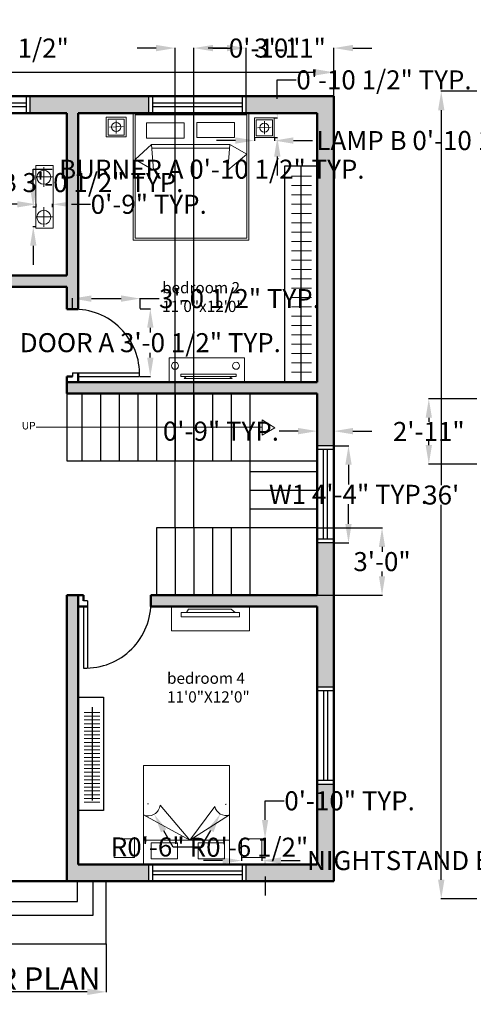
# Model space of a CAD drawing. Units: inches. Extents: x 18 to 9768, y 4 to 3529.
# Tile 3 of 6: x 9006 to 9249, y 3002 to 3529. Entities that reach past the tile are written whole.
import ezdxf

# ---------------------------------------------------------------- set-up
doc = ezdxf.new("R2010")
doc.units = ezdxf.units.IN
doc.header["$MEASUREMENT"] = 0
for name, color, linetype, lineweight in [('A-ANNO-DIMS', 2, 'Continuous', 18), ('A-ANNO-SYMB', 2, 'Continuous', 18), ('A-ANNO-TEXT', 7, 'Continuous', 25), ('A-AREA-IDEN', 7, 'Continuous', 18), ('A-CASE-PATT', 9, 'Continuous', 13), ('A-EQPM', 8, 'Continuous', 18), ('A-FLOR-CASE', 9, 'Continuous', 25), ('A-FLOR-STRS', 7, 'Continuous', 25), ('A-FURN', 8, 'Continuous', 18), ('A-WALL-PATT', 252, 'Continuous', 13), ('WAL', 7, 'Continuous', 50)]:
    doc.layers.add(name, color=color, linetype=linetype, lineweight=lineweight)
doc.layers.add('A-DOOR', color=30, linetype='Continuous', lineweight=25, true_color=0xf8991e)
doc.layers.add('A-GLAZ', color=177, linetype='Continuous', lineweight=25, true_color=0x293189)
doc.styles.get("Standard").update_dxf_attribs({"font": 'arial.ttf'})
doc.dimstyles.get("Standard").update_dxf_attribs({"dimtxt": 10.18, "dimasz": 10.18, "dimexe": 0.18, "dimexo": 0.0625, "dimgap": 0.09, "dimtad": 0, "dimtih": 1, "dimtoh": 1, "dimdec": 0, "dimzin": 0, "dimdsep": 46, "dimlunit": 3, "dimtxsty": 'Standard', "dimcen": 0.09, "dimadec": 0, "dimazin": 0, "dimtfac": 1, "dimtdec": 0, "dimtofl": 0, "dimtmove": 0, "dimatfit": 3, "dimfxl": 1, "dimtolj": 1, "dimtzin": 0, "dimarcsym": 0})

# ---------------------------------------------------------------- blocks, each defined once
blk = doc.blocks.new('*D3')
at = {"layer": 'A-ANNO-DIMS', "color": 0, "lineweight": -2, "transparency": 16777216}
for p, q in [((8753.89, 3487.8), (8753.89, 3500.68)), ((8764.07, 3500.5), (8955.16, 3500.5)), ((9163.71, 3500.5), (8972.61, 3500.5)), ((9173.89, 3487.8), (9173.89, 3500.68))]:
    blk.add_line(p, q, dxfattribs=at)
at = {"layer": 'A-ANNO-DIMS', "color": 0, "transparency": 16777216}
for points in [[(8764.07, 3502.19), (8764.07, 3498.8), (8753.89, 3500.5)], [(9163.71, 3502.19), (9163.71, 3498.8), (9173.89, 3500.5)]]:
    blk.add_solid(points, dxfattribs=at)
at = {"layer": 'Defpoints', "color": 0, "transparency": 16777216}
for p in [(9173.89, 3500.5), (8753.89, 3487.73), (9173.89, 3487.73)]:
    blk.add_point(p, dxfattribs=at)
at = {"layer": 'A-ANNO-DIMS', "color": 0, "transparency": 16777216, "insert": (8963.89, 3500.5), "char_height": 10.18, "attachment_point": 5}
blk.add_mtext("\\A1;35'", dxfattribs=at)
blk = doc.blocks.new('*D8')
at = {"layer": 'A-ANNO-DIMS', "color": 0, "lineweight": -2, "transparency": 16777216}
for p, q in [((9250.37, 3490.36), (9231.16, 3490.36)), ((9231.34, 3480.18), (9231.34, 3279.65)), ((9231.34, 3068.54), (9231.34, 3269.07)), ((9250.37, 3058.36), (9231.16, 3058.36))]:
    blk.add_line(p, q, dxfattribs=at)
at = {"layer": 'A-ANNO-DIMS', "color": 0, "transparency": 16777216}
for points in [[(9229.65, 3480.18), (9233.04, 3480.18), (9231.34, 3490.36)], [(9229.65, 3068.54), (9233.04, 3068.54), (9231.34, 3058.36)]]:
    blk.add_solid(points, dxfattribs=at)
at = {"layer": 'Defpoints', "color": 0, "transparency": 16777216}
for p in [(9250.43, 3490.36), (9231.34, 3058.36), (9250.43, 3058.36)]:
    blk.add_point(p, dxfattribs=at)
at = {"layer": 'A-ANNO-DIMS', "color": 0, "transparency": 16777216, "insert": (9231.34, 3274.36), "char_height": 10.18, "attachment_point": 5}
blk.add_mtext("\\A1;36'", dxfattribs=at)
blk = doc.blocks.new('WINDOW-48')
for p, q in [((0, 0), (0, 9)), ((2, 0), (2, 9)), ((2, 5.5), (50, 5.5)), ((50, 0), (50, 9)), ((52, 0), (52, 9)), ((2, 3.5), (50, 3.5))]:
    blk.add_line(p, q)
blk = doc.blocks.new('DOOR-36-W6')
for p, q in [((34.01, 0), (34.01, 36)), ((36.01, 3), (36.01, 36)), ((34.01, 0), (36.01, 0))]:
    blk.add_line(p, q)
blk.add_arc((35.01, 1), 35.01, 88.3634, 181.6366)
blk = doc.blocks.new('NIGHTSTAND-LAMP-B')
for p, q in [((1.67, 5.25), (8.97, 5.48)), ((5.32, 8.7), (5.32, 1.86))]:
    blk.add_line(p, q)
for points in [[(0, 10.5), (10.63, 10.5), (10.63, 0), (0, 0)], [(1, 9.5), (9.63, 9.5), (9.63, 1), (1, 1)]]:
    blk.add_lwpolyline(points, close=True)
blk.add_circle((5.32, 5.25), 2.45)
blk = doc.blocks.new('COOKTOP-BURNER-7')
for p, q in [((0, 5.3), (8.79, 5.3)), ((4.14, 10.42), (4.14, 0))]:
    blk.add_line(p, q)
blk.add_circle((4.08, 5.04), 3.73)
blk = doc.blocks.new('NIGHTSTAND-SMALL')
blk.add_lwpolyline([(0, 9.97), (10.94, 9.97), (10.94, 0), (0, 0)], close=True)
blk = doc.blocks.new('*D25')
at = {"layer": 'A-ANNO-DIMS', "color": 0, "lineweight": -2, "transparency": 16777216}
for p, q in [((9173.95, 3300.73), (9181.87, 3300.73)), ((9181.69, 3290.55), (9181.69, 3279.94)), ((9181.69, 3258.91), (9181.69, 3269.53)), ((9173.95, 3248.73), (9181.87, 3248.73))]:
    blk.add_line(p, q, dxfattribs=at)
at = {"layer": 'A-ANNO-DIMS', "color": 0, "transparency": 16777216}
for points in [[(9179.99, 3290.55), (9183.38, 3290.55), (9181.69, 3300.73)], [(9179.99, 3258.91), (9183.38, 3258.91), (9181.69, 3248.73)]]:
    blk.add_solid(points, dxfattribs=at)
at = {"layer": 'Defpoints', "color": 0, "transparency": 16777216}
for p in [(9173.89, 3300.73), (9181.69, 3300.73), (9173.89, 3248.73)]:
    blk.add_point(p, dxfattribs=at)
at = {"layer": 'A-ANNO-DIMS', "color": 0, "transparency": 16777216, "insert": (9181.69, 3274.73), "char_height": 10.18, "attachment_point": 5}
blk.add_mtext('\\A1;W1 4\'-4" TYP.', dxfattribs=at)
blk = doc.blocks.new('*D26')
at = {"layer": 'A-ANNO-DIMS', "color": 0, "lineweight": -2, "transparency": 16777216}
for p, q in [((9154.71, 3308.53), (9144.53, 3308.53)), ((9164.89, 3300.8), (9164.89, 3308.71)), ((9173.89, 3300.8), (9173.89, 3308.71)), ((9184.07, 3308.53), (9194.25, 3308.53))]:
    blk.add_line(p, q, dxfattribs=at)
at = {"layer": 'A-ANNO-DIMS', "color": 0, "transparency": 16777216}
for points in [[(9154.71, 3310.23), (9154.71, 3306.84), (9164.89, 3308.53)], [(9184.07, 3310.23), (9184.07, 3306.84), (9173.89, 3308.53)]]:
    blk.add_solid(points, dxfattribs=at)
at = {"layer": 'Defpoints', "color": 0, "transparency": 16777216}
for p in [(9164.89, 3308.53), (9164.89, 3300.73), (9173.89, 3300.73)]:
    blk.add_point(p, dxfattribs=at)
at = {"layer": 'A-ANNO-DIMS', "color": 0, "transparency": 16777216, "insert": (9113.41, 3308.53), "char_height": 10.18, "attachment_point": 5}
blk.add_mtext('\\A1;0\'-9" TYP.', dxfattribs=at)
blk = doc.blocks.new('*D29')
at = {"layer": 'A-ANNO-DIMS', "color": 0, "lineweight": -2, "transparency": 16777216}
for p, q in [((9070.22, 3374.01), (9075.78, 3374.01)), ((9075.6, 3363.83), (9075.6, 3361.23)), ((9075.6, 3347.91), (9075.6, 3350.51)), ((9070.22, 3337.73), (9075.78, 3337.73))]:
    blk.add_line(p, q, dxfattribs=at)
at = {"layer": 'A-ANNO-DIMS', "color": 0, "transparency": 16777216}
for points in [[(9073.9, 3363.83), (9077.3, 3363.83), (9075.6, 3374.01)], [(9073.9, 3347.91), (9077.3, 3347.91), (9075.6, 3337.73)]]:
    blk.add_solid(points, dxfattribs=at)
at = {"layer": 'Defpoints', "color": 0, "transparency": 16777216}
for p in [(9070.16, 3374.01), (9070.16, 3337.73), (9075.6, 3337.73)]:
    blk.add_point(p, dxfattribs=at)
at = {"layer": 'A-ANNO-DIMS', "color": 0, "transparency": 16777216, "insert": (9075.6, 3355.87), "char_height": 10.18, "attachment_point": 5}
blk.add_mtext('\\A1;DOOR A 3\'-0 1/2" TYP.', dxfattribs=at)
blk = doc.blocks.new('*D30')
at = {"layer": 'A-ANNO-DIMS', "color": 0, "lineweight": -2, "transparency": 16777216}
for p, q in [((9033.89, 3374.07), (9033.89, 3379.63)), ((9044.07, 3379.45), (9059.98, 3379.45)), ((9070.16, 3374.07), (9070.16, 3379.63)), ((9070.16, 3379.45), (9080.34, 3379.45))]:
    blk.add_line(p, q, dxfattribs=at)
at = {"layer": 'A-ANNO-DIMS', "color": 0, "transparency": 16777216}
for points in [[(9044.07, 3381.15), (9044.07, 3377.75), (9033.89, 3379.45)], [(9059.98, 3381.15), (9059.98, 3377.75), (9070.16, 3379.45)]]:
    blk.add_solid(points, dxfattribs=at)
at = {"layer": 'Defpoints', "color": 0, "transparency": 16777216}
for p in [(9070.16, 3379.45), (9033.89, 3374.01), (9070.16, 3374.01)]:
    blk.add_point(p, dxfattribs=at)
at = {"layer": 'A-ANNO-DIMS', "color": 0, "transparency": 16777216, "insert": (9123.31, 3379.45), "char_height": 10.18, "attachment_point": 5}
blk.add_mtext('\\A1;3\'-0 1/2" TYP.', dxfattribs=at)
blk = doc.blocks.new('*D31')
at = {"layer": 'A-ANNO-DIMS', "color": 0, "lineweight": -2, "transparency": 16777216}
for p, q in [((8903.89, 3446.9), (8903.89, 3441.34)), ((8940.16, 3446.9), (8940.16, 3441.34)), ((8914.07, 3441.52), (8929.98, 3441.52)), ((8940.16, 3441.52), (8950.34, 3441.52))]:
    blk.add_line(p, q, dxfattribs=at)
at = {"layer": 'A-ANNO-DIMS', "color": 0, "transparency": 16777216}
for points in [[(8914.07, 3443.21), (8914.07, 3439.82), (8903.89, 3441.52)], [(8929.98, 3443.21), (8929.98, 3439.82), (8940.16, 3441.52)]]:
    blk.add_solid(points, dxfattribs=at)
at = {"layer": 'Defpoints', "color": 0, "transparency": 16777216}
for p in [(8903.89, 3446.96), (8940.16, 3446.96), (8940.16, 3441.52)]:
    blk.add_point(p, dxfattribs=at)
at = {"layer": 'A-ANNO-DIMS', "color": 0, "transparency": 16777216, "insert": (9023.09, 3441.52), "char_height": 10.18, "attachment_point": 5}
blk.add_mtext('\\A1;DOOR B 3\'-0 1/2" TYP.', dxfattribs=at)
blk = doc.blocks.new('*D41')
at = {"layer": 'A-ANNO-DIMS', "color": 0, "lineweight": -2, "transparency": 16777216}
for p, q in [((9012.94, 3438.5), (9012.94, 3448.68)), ((9012.94, 3448.68), (9023.12, 3448.68)), ((9014.44, 3428.32), (9012.76, 3428.32)), ((9014.44, 3417.91), (9012.76, 3417.91)), ((9012.94, 3407.73), (9012.94, 3397.55))]:
    blk.add_line(p, q, dxfattribs=at)
at = {"layer": 'A-ANNO-DIMS', "color": 0, "transparency": 16777216}
for points in [[(9011.24, 3438.5), (9014.63, 3438.5), (9012.94, 3428.32)], [(9011.24, 3407.73), (9014.63, 3407.73), (9012.94, 3417.91)]]:
    blk.add_solid(points, dxfattribs=at)
at = {"layer": 'Defpoints', "color": 0, "transparency": 16777216}
for p in [(9012.94, 3428.32), (9014.5, 3428.32), (9014.5, 3417.91)]:
    blk.add_point(p, dxfattribs=at)
at = {"layer": 'A-ANNO-DIMS', "color": 0, "transparency": 16777216, "insert": (9108.54, 3448.68), "char_height": 10.18, "attachment_point": 5}
blk.add_mtext('\\A1;BURNER A 0\'-10 1/2" TYP.', dxfattribs=at)
blk = doc.blocks.new('*D42')
at = {"layer": 'A-ANNO-DIMS', "color": 0, "lineweight": -2, "transparency": 16777216}
for p, q in [((9004.32, 3429.89), (8994.14, 3429.89)), ((9014.5, 3428.39), (9014.5, 3430.07)), ((9023.29, 3428.39), (9023.29, 3430.07)), ((9033.47, 3429.89), (9043.65, 3429.89))]:
    blk.add_line(p, q, dxfattribs=at)
at = {"layer": 'A-ANNO-DIMS', "color": 0, "transparency": 16777216}
for points in [[(9004.32, 3431.58), (9004.32, 3428.19), (9014.5, 3429.89)], [(9033.47, 3431.58), (9033.47, 3428.19), (9023.29, 3429.89)]]:
    blk.add_solid(points, dxfattribs=at)
at = {"layer": 'Defpoints', "color": 0, "transparency": 16777216}
for p in [(9023.29, 3429.89), (9014.5, 3428.32), (9023.29, 3428.32)]:
    blk.add_point(p, dxfattribs=at)
at = {"layer": 'A-ANNO-DIMS', "color": 0, "transparency": 16777216, "insert": (9074.76, 3429.89), "char_height": 10.18, "attachment_point": 5}
blk.add_mtext('\\A1;0\'-9" TYP.', dxfattribs=at)
blk = doc.blocks.new('*D49')
at = {"layer": 'A-ANNO-DIMS', "color": 0, "lineweight": -2, "transparency": 16777216}
for p, q in [((9121.17, 3464.01), (9110.99, 3464.01)), ((9131.35, 3465.54), (9131.35, 3463.83)), ((9141.99, 3465.54), (9141.99, 3463.83)), ((9152.17, 3464.01), (9162.35, 3464.01))]:
    blk.add_line(p, q, dxfattribs=at)
at = {"layer": 'A-ANNO-DIMS', "color": 0, "transparency": 16777216}
for points in [[(9121.17, 3465.71), (9121.17, 3462.32), (9131.35, 3464.01)], [(9152.17, 3465.71), (9152.17, 3462.32), (9141.99, 3464.01)]]:
    blk.add_solid(points, dxfattribs=at)
at = {"layer": 'Defpoints', "color": 0, "transparency": 16777216}
for p in [(9131.35, 3465.61), (9141.99, 3465.61), (9141.99, 3464.01)]:
    blk.add_point(p, dxfattribs=at)
at = {"layer": 'A-ANNO-DIMS', "color": 0, "transparency": 16777216, "insert": (9237.11, 3464.01), "char_height": 10.18, "attachment_point": 5}
blk.add_mtext('\\A1;LAMP B 0\'-10 1/2" TYP.', dxfattribs=at)
blk = doc.blocks.new('*D50')
at = {"layer": 'A-ANNO-DIMS', "color": 0, "lineweight": -2, "transparency": 16777216}
for p, q in [((9143.58, 3486.29), (9143.58, 3496.47)), ((9143.58, 3496.47), (9153.76, 3496.47)), ((9142.05, 3476.11), (9143.76, 3476.11)), ((9142.05, 3465.61), (9143.76, 3465.61)), ((9143.58, 3455.43), (9143.58, 3445.25))]:
    blk.add_line(p, q, dxfattribs=at)
at = {"layer": 'A-ANNO-DIMS', "color": 0, "transparency": 16777216}
for points in [[(9141.89, 3486.29), (9145.28, 3486.29), (9143.58, 3476.11)], [(9141.89, 3455.43), (9145.28, 3455.43), (9143.58, 3465.61)]]:
    blk.add_solid(points, dxfattribs=at)
at = {"layer": 'Defpoints', "color": 0, "transparency": 16777216}
for p in [(9141.99, 3476.11), (9143.58, 3476.11), (9141.99, 3465.61)]:
    blk.add_point(p, dxfattribs=at)
at = {"layer": 'A-ANNO-DIMS', "color": 0, "transparency": 16777216, "insert": (9200.69, 3496.47), "char_height": 10.18, "attachment_point": 5}
blk.add_mtext('\\A1;0\'-10 1/2" TYP.', dxfattribs=at)
blk = doc.blocks.new('*D55')
at = {"layer": 'A-ANNO-DIMS', "color": 0, "lineweight": -2, "transparency": 16777216}
for p, q in [((9114.26, 3078.78), (9104.08, 3078.78)), ((9124.44, 3080.36), (9124.44, 3078.6)), ((9135.38, 3080.36), (9135.38, 3078.6)), ((9145.56, 3078.78), (9155.74, 3078.78))]:
    blk.add_line(p, q, dxfattribs=at)
at = {"layer": 'A-ANNO-DIMS', "color": 0, "transparency": 16777216}
for points in [[(9114.26, 3080.48), (9114.26, 3077.09), (9124.44, 3078.78)], [(9145.56, 3080.48), (9145.56, 3077.09), (9135.38, 3078.78)]]:
    blk.add_solid(points, dxfattribs=at)
at = {"layer": 'Defpoints', "color": 0, "transparency": 16777216}
for p in [(9124.44, 3080.42), (9135.38, 3080.42), (9135.38, 3078.78)]:
    blk.add_point(p, dxfattribs=at)
at = {"layer": 'A-ANNO-DIMS', "color": 0, "transparency": 16777216, "insert": (9245.48, 3078.78), "char_height": 10.18, "attachment_point": 5}
blk.add_mtext('\\A1;NIGHTSTAND B 0\'-11" TYP.', dxfattribs=at)
blk = doc.blocks.new('*D56')
at = {"layer": 'A-ANNO-DIMS', "color": 0, "lineweight": -2, "transparency": 16777216}
for p, q in [((9137.02, 3100.57), (9137.02, 3110.75)), ((9137.02, 3110.75), (9147.2, 3110.75)), ((9135.44, 3090.39), (9137.2, 3090.39)), ((9135.44, 3080.42), (9137.2, 3080.42)), ((9137.02, 3070.24), (9137.02, 3060.06))]:
    blk.add_line(p, q, dxfattribs=at)
at = {"layer": 'A-ANNO-DIMS', "color": 0, "transparency": 16777216}
for points in [[(9135.33, 3100.57), (9138.72, 3100.57), (9137.02, 3090.39)], [(9135.33, 3070.24), (9138.72, 3070.24), (9137.02, 3080.42)]]:
    blk.add_solid(points, dxfattribs=at)
at = {"layer": 'Defpoints', "color": 0, "transparency": 16777216}
for p in [(9135.38, 3090.39), (9137.02, 3090.39), (9135.38, 3080.42)]:
    blk.add_point(p, dxfattribs=at)
at = {"layer": 'A-ANNO-DIMS', "color": 0, "transparency": 16777216, "insert": (9182.27, 3110.75), "char_height": 10.18, "attachment_point": 5}
blk.add_mtext('\\A1;0\'-10" TYP.', dxfattribs=at)
blk = doc.blocks.new('*D57')
at = {"layer": 'A-ANNO-DIMS', "color": 0, "lineweight": -2, "transparency": 16777216}
for p, q in [((8882.05, 3034.24), (8882.05, 3008.38)), ((9052.03, 3034.24), (9052.03, 3008.38)), ((8892.23, 3008.56), (8949.95, 3008.56)), ((9041.85, 3008.56), (8984.14, 3008.56))]:
    blk.add_line(p, q, dxfattribs=at)
at = {"layer": 'A-ANNO-DIMS', "color": 0, "transparency": 16777216}
for points in [[(8892.23, 3010.25), (8892.23, 3006.86), (8882.05, 3008.56)], [(9041.85, 3010.25), (9041.85, 3006.86), (9052.03, 3008.56)]]:
    blk.add_solid(points, dxfattribs=at)
at = {"layer": 'Defpoints', "color": 0, "transparency": 16777216}
for p in [(8882.05, 3034.31), (9052.03, 3034.31), (9052.03, 3008.56)]:
    blk.add_point(p, dxfattribs=at)
at = {"layer": 'A-ANNO-DIMS', "color": 0, "transparency": 16777216, "insert": (8967.04, 3008.56), "char_height": 10.18, "attachment_point": 5}
blk.add_mtext('\\A1;14\'-2"', dxfattribs=at)
blk = doc.blocks.new('*D61')
at = {"layer": 'A-ANNO-DIMS', "color": 0, "lineweight": -2, "transparency": 16777216}
for p, q in [((9164.95, 3256.73), (9199.82, 3256.73)), ((9199.64, 3246.55), (9199.64, 3244.03)), ((9199.64, 3230.91), (9199.64, 3233.44)), ((9164.95, 3220.73), (9199.82, 3220.73))]:
    blk.add_line(p, q, dxfattribs=at)
at = {"layer": 'A-ANNO-DIMS', "color": 0, "transparency": 16777216}
for points in [[(9197.94, 3246.55), (9201.33, 3246.55), (9199.64, 3256.73)], [(9197.94, 3230.91), (9201.33, 3230.91), (9199.64, 3220.73)]]:
    blk.add_solid(points, dxfattribs=at)
at = {"layer": 'Defpoints', "color": 0, "transparency": 16777216}
for p in [(9164.89, 3256.73), (9199.64, 3256.73), (9164.89, 3220.73)]:
    blk.add_point(p, dxfattribs=at)
at = {"layer": 'A-ANNO-DIMS', "color": 0, "transparency": 16777216, "insert": (9199.64, 3238.73), "char_height": 10.18, "attachment_point": 5}
blk.add_mtext('\\A1;3\'-0"', dxfattribs=at)
blk = doc.blocks.new('*D62')
at = {"layer": 'A-ANNO-DIMS', "color": 0, "lineweight": -2, "transparency": 16777216}
for p, q in [((9078.71, 3513.48), (9068.53, 3513.48)), ((9088.89, 3256.8), (9088.89, 3513.66)), ((9098.89, 3256.8), (9098.89, 3513.66)), ((9109.07, 3513.48), (9119.25, 3513.48))]:
    blk.add_line(p, q, dxfattribs=at)
at = {"layer": 'A-ANNO-DIMS', "color": 0, "transparency": 16777216}
for points in [[(9078.71, 3515.18), (9078.71, 3511.79), (9088.89, 3513.48)], [(9109.07, 3515.18), (9109.07, 3511.79), (9098.89, 3513.48)]]:
    blk.add_solid(points, dxfattribs=at)
at = {"layer": 'Defpoints', "color": 0, "transparency": 16777216}
for p in [(9098.89, 3513.48), (9088.89, 3256.73), (9098.89, 3256.73)]:
    blk.add_point(p, dxfattribs=at)
at = {"layer": 'A-ANNO-DIMS', "color": 0, "transparency": 16777216, "insert": (9136.82, 3513.48), "char_height": 10.18, "attachment_point": 5}
blk.add_mtext('\\A1;0\'-10"', dxfattribs=at)
blk = doc.blocks.new('*D70')
at = {"layer": 'A-ANNO-DIMS', "color": 0, "lineweight": -2, "transparency": 16777216}
for p, q in [((8929.71, 3513.48), (8919.53, 3513.48)), ((8939.89, 3487.8), (8939.89, 3513.66)), ((8959.3, 3487.8), (8959.3, 3513.66)), ((8969.48, 3513.48), (8979.66, 3513.48))]:
    blk.add_line(p, q, dxfattribs=at)
at = {"layer": 'A-ANNO-DIMS', "color": 0, "transparency": 16777216}
for points in [[(8929.71, 3515.18), (8929.71, 3511.79), (8939.89, 3513.48)], [(8969.48, 3515.18), (8969.48, 3511.79), (8959.3, 3513.48)]]:
    blk.add_solid(points, dxfattribs=at)
at = {"layer": 'Defpoints', "color": 0, "transparency": 16777216}
for p in [(8959.3, 3513.48), (8939.89, 3487.73), (8959.3, 3487.73)]:
    blk.add_point(p, dxfattribs=at)
at = {"layer": 'A-ANNO-DIMS', "color": 0, "transparency": 16777216, "insert": (9004.67, 3513.48), "char_height": 10.18, "attachment_point": 5}
blk.add_mtext('\\A1;1\'-7 1/2"', dxfattribs=at)
blk = doc.blocks.new('*D71')
at = {"layer": 'A-ANNO-DIMS', "color": 0, "lineweight": -2, "transparency": 16777216}
for p, q in [((9116.71, 3513.48), (9106.53, 3513.48)), ((9126.89, 3487.8), (9126.89, 3513.66)), ((9173.89, 3487.8), (9173.89, 3513.66)), ((9184.07, 3513.48), (9194.25, 3513.48))]:
    blk.add_line(p, q, dxfattribs=at)
at = {"layer": 'A-ANNO-DIMS', "color": 0, "transparency": 16777216}
for points in [[(9116.71, 3515.18), (9116.71, 3511.79), (9126.89, 3513.48)], [(9184.07, 3515.18), (9184.07, 3511.79), (9173.89, 3513.48)]]:
    blk.add_solid(points, dxfattribs=at)
at = {"layer": 'Defpoints', "color": 0, "transparency": 16777216}
for p in [(9173.89, 3513.48), (9126.89, 3487.73), (9173.89, 3487.73)]:
    blk.add_point(p, dxfattribs=at)
at = {"layer": 'A-ANNO-DIMS', "color": 0, "transparency": 16777216, "insert": (9150.39, 3513.48), "char_height": 10.18, "attachment_point": 5}
blk.add_mtext('\\A1;3\'-11"', dxfattribs=at)
blk = doc.blocks.new('*D78')
at = {"layer": 'A-ANNO-DIMS', "color": 0, "lineweight": -2, "transparency": 16777216}
for p, q in [((9250.37, 3325.86), (9224.5, 3325.86)), ((9224.68, 3315.68), (9224.68, 3313.56)), ((9224.68, 3301.04), (9224.68, 3303.16)), ((9250.37, 3290.86), (9224.5, 3290.86))]:
    blk.add_line(p, q, dxfattribs=at)
at = {"layer": 'A-ANNO-DIMS', "color": 0, "transparency": 16777216}
for points in [[(9222.99, 3315.68), (9226.38, 3315.68), (9224.68, 3325.86)], [(9222.99, 3301.04), (9226.38, 3301.04), (9224.68, 3290.86)]]:
    blk.add_solid(points, dxfattribs=at)
at = {"layer": 'Defpoints', "color": 0, "transparency": 16777216}
for p in [(9224.68, 3325.86), (9250.43, 3325.86), (9250.43, 3290.86)]:
    blk.add_point(p, dxfattribs=at)
at = {"layer": 'A-ANNO-DIMS', "color": 0, "transparency": 16777216, "insert": (9224.68, 3308.36), "char_height": 10.18, "attachment_point": 5}
blk.add_mtext('\\A1;2\'-11"', dxfattribs=at)
blk = doc.blocks.new('*D90')
at = {"layer": 'A-ANNO-DIMS', "color": 0, "lineweight": -2, "transparency": 16777216}
for p, q in [((9074.33, 3109.21), (9074.51, 3109.21)), ((9074.42, 3109.12), (9074.42, 3109.3)), ((9087.87, 3085.92), (9082.78, 3094.73)), ((9098.05, 3085.92), (9087.87, 3085.92))]:
    blk.add_line(p, q, dxfattribs=at)
at = {"layer": 'A-ANNO-DIMS', "color": 0, "transparency": 16777216}
blk.add_solid([(9084.25, 3095.58), (9081.31, 3093.88), (9077.69, 3103.55)], dxfattribs=at)
at = {"layer": 'Defpoints', "color": 0, "transparency": 16777216}
for p in [(9074.42, 3109.21), (9077.69, 3103.55)]:
    blk.add_point(p, dxfattribs=at)
at = {"layer": 'A-ANNO-DIMS', "color": 0, "transparency": 16777216, "insert": (9128.4, 3085.92), "char_height": 10.18, "attachment_point": 5}
blk.add_mtext('\\A1;R0\'-6 1/2"', dxfattribs=at)
blk = doc.blocks.new('*D91')
at = {"layer": 'A-ANNO-DIMS', "color": 0, "lineweight": -2, "transparency": 16777216}
for p, q in [((9115.98, 3108.92), (9116.16, 3108.92)), ((9116.07, 3108.83), (9116.07, 3109.01)), ((9102.87, 3086.06), (9107.96, 3094.87)), ((9092.69, 3086.06), (9102.87, 3086.06))]:
    blk.add_line(p, q, dxfattribs=at)
at = {"layer": 'A-ANNO-DIMS', "color": 0, "transparency": 16777216}
blk.add_solid([(9106.49, 3095.72), (9109.43, 3094.02), (9113.05, 3103.69)], dxfattribs=at)
at = {"layer": 'Defpoints', "color": 0, "transparency": 16777216}
for p in [(9116.07, 3108.92), (9113.05, 3103.69)]:
    blk.add_point(p, dxfattribs=at)
at = {"layer": 'A-ANNO-DIMS', "color": 0, "transparency": 16777216, "insert": (9074.2, 3086.06), "char_height": 10.18, "attachment_point": 5}
blk.add_mtext('\\A1;R0\'-6"', dxfattribs=at)

msp = doc.modelspace()

# ---------------------------------------------------------------- hatches: boundary and pattern name
at = {"layer": 'A-CASE-PATT'}
h = msp.add_hatch(dxfattribs=at)
h.set_pattern_fill('ANSI31', color=256, scale=40, angle=-45, style=0)
h.paths.add_polyline_path([(9151.25, 3338.01), (9161.82, 3338.01), (9161.82, 3448.01), (9151.25, 3448.01)])
h = msp.add_hatch(dxfattribs=at)
h.set_pattern_fill('ANSI31', color=256, scale=16, angle=-45, style=0)
h.paths.add_polyline_path([(9040.16, 3109.7), (9048.51, 3109.7), (9048.51, 3159.7), (9040.16, 3159.7)])
at = {"layer": 'A-WALL-PATT'}
h = msp.add_hatch(color=256, dxfattribs=at)
h.dxf.hatch_style = 1
h.paths.add_polyline_path([(8762.89, 3478.73), (8802.89, 3478.73), (8802.89, 3487.73), (8753.89, 3487.73), (8753.89, 3317.23), (8762.89, 3317.23), (8762.89, 3328.73), (8813.89, 3328.73), (8813.89, 3329.73, -0.017236), (8813.89, 3331.73), (8813.89, 3334.73), (8762.89, 3334.73)])
h.paths.add_polyline_path([(8900.89, 3487.73), (8854.89, 3487.73), (8854.89, 3478.73), (8894.89, 3478.73), (8894.89, 3421.46), (8894.89, 3334.73), (8894.89, 3328.73), (8900.89, 3328.73), (8900.89, 3391.73), (8900.89, 3478.73)])
h.paths.add_polyline_path([(9074.89, 3487.73), (9011.3, 3487.73), (9011.3, 3478.73), (9030.89, 3478.73), (9030.89, 3391.73), (8939.89, 3391.73), (8939.89, 3390.73, -0.014283), (8939.89, 3388.73), (8939.89, 3385.73), (9030.89, 3385.73), (9030.89, 3373.73), (9033.89, 3373.73, -0.014283), (9035.89, 3373.73), (9036.89, 3373.73), (9036.89, 3478.73), (9074.89, 3478.73)])
h.paths.add_polyline_path([(9173.89, 3487.73), (9126.89, 3487.73), (9126.89, 3478.73), (9128.34, 3478.73), (9164.89, 3478.73), (9164.89, 3334.73), (9147.51, 3334.73), (9036.89, 3334.73), (9030.89, 3334.73), (9030.89, 3328.73), (9164.89, 3328.73), (9164.89, 3300.73), (9173.89, 3300.73)])
h.paths.add_polyline_path([(8762.89, 3271.73), (8846.89, 3271.73), (8852.89, 3271.73), (8852.89, 3328.73), (8855.89, 3328.73), (8855.89, 3331.73, -0.014283), (8855.89, 3333.73), (8855.89, 3334.73), (8846.89, 3334.73), (8846.89, 3328.73), (8846.89, 3277.73), (8762.89, 3277.73), (8762.89, 3289.23), (8753.89, 3289.23), (8753.89, 3260.23), (8762.89, 3260.23)])
h.paths.add_polyline_path([(8762.89, 3214.73), (8855.89, 3214.73), (8855.89, 3215.73, -0.014283), (8855.89, 3217.73), (8855.89, 3220.73), (8852.89, 3220.73), (8852.89, 3238.73), (8849.89, 3238.73, -0.017236), (8847.89, 3238.73), (8846.89, 3238.73), (8846.89, 3220.73), (8762.89, 3220.73), (8762.89, 3232.23), (8753.89, 3232.23), (8753.89, 3171.73), (8762.89, 3171.73)])
h.paths.add_polyline_path([(8762.89, 3119.73), (8753.89, 3119.73), (8753.89, 3067.73), (8802.89, 3067.73), (8802.89, 3076.73), (8795.03, 3076.73), (8762.89, 3076.73)])
h.paths.add_polyline_path([(8900.89, 3076.73), (8900.89, 3214.73), (8987.37, 3214.73), (8987.37, 3220.73), (8894.89, 3220.73), (8894.89, 3214.73), (8894.89, 3076.73), (8854.89, 3076.73), (8854.89, 3067.73), (8900.89, 3067.73)])
h.paths.add_polyline_path([(9074.89, 3076.73), (9071.87, 3076.73), (9036.89, 3076.73), (9036.89, 3214.73), (9036.89, 3220.73), (9030.89, 3220.73), (9030.89, 3214.73), (9030.89, 3076.73), (9030.89, 3067.73), (9074.89, 3067.73)])
h.paths.add_polyline_path([(9173.89, 3119.73), (9164.89, 3119.73), (9164.89, 3076.73), (9126.89, 3076.73), (9126.89, 3067.73), (9173.89, 3067.73)])
h.paths.add_polyline_path([(9173.89, 3248.73), (9164.89, 3248.73), (9164.89, 3220.73), (9075.89, 3220.73), (9075.89, 3217.73, -0.014283), (9075.89, 3215.73), (9075.89, 3214.73), (9164.89, 3214.73), (9164.89, 3171.73), (9173.89, 3171.73)])

# ---------------------------------------------------------------- linework, layer by layer
at = {"layer": 'A-ANNO-SYMB'}
for p, q in [((9135.43, 3310.73), (9135.43, 3314.63)), ((9135.43, 3314.63), (9135.43, 3306.38)), ((9142.34, 3310.37), (9135.43, 3314.63)), ((9014.54, 3310.73), (9135.43, 3310.73)), ((9135.43, 3306.38), (9142.34, 3310.37))]:
    msp.add_line(p, q, dxfattribs=at)
at = {"layer": 'A-EQPM'}
for p, q in [((9094.83, 3337.8), (9093.8, 3336.72)), ((9093.8, 3336.72), (9119.49, 3336.72)), ((9119.49, 3336.72), (9117.95, 3337.8)), ((9095.02, 3211.57), (9096.03, 3213.24)), ((9096.03, 3213.24), (9118.9, 3213.24)), ((9118.9, 3213.24), (9121.01, 3211.57))]:
    msp.add_line(p, q, dxfattribs=at)
for points in [[(9014.32, 3450.74), (9023.55, 3450.74), (9023.55, 3417.19), (9014.32, 3417.19)], [(9085.77, 3334.73), (9126.04, 3334.73), (9126.04, 3347.71), (9085.77, 3347.71)], [(9091.86, 3339.04), (9121.56, 3339.04), (9121.56, 3337.8), (9091.86, 3337.8)], [(9086.96, 3214.73), (9128.63, 3214.73), (9128.63, 3201.74), (9086.96, 3201.74)], [(9092.09, 3211.57), (9123.28, 3211.57), (9123.28, 3209.24), (9092.09, 3209.24)]]:
    msp.add_lwpolyline(points, close=True, dxfattribs=at)
for centre in [(9088.8, 3343.51), (9121.5, 3343.51)]:
    msp.add_circle(centre, 1.9, dxfattribs=at)
at = {"layer": 'A-FLOR-CASE'}
for p, q in [((9156.2, 3450.38), (9156.2, 3334.73)), ((9044.55, 3160.87), (9044.55, 3110.83))]:
    msp.add_line(p, q, dxfattribs=at)
for points in [[(9164.89, 3450.38), (9147.51, 3450.38), (9147.51, 3334.73), (9164.89, 3334.73)], [(9036.89, 3166.22), (9050.55, 3166.22), (9050.55, 3105.63), (9036.89, 3105.63)]]:
    msp.add_lwpolyline(points, close=True, dxfattribs=at)
at = {"layer": 'A-FLOR-STRS'}
for p, q in [((9030.89, 3328.73), (9030.89, 3292.73)), ((9038.89, 3328.73), (9038.89, 3292.73)), ((9048.89, 3328.73), (9048.89, 3292.73)), ((9058.89, 3328.73), (9058.89, 3292.73)), ((9068.89, 3328.73), (9068.89, 3292.73)), ((9078.89, 3328.73), (9078.89, 3292.73)), ((9088.89, 3328.73), (9088.89, 3292.73)), ((9098.89, 3328.73), (9098.89, 3292.73)), ((9108.89, 3328.73), (9108.89, 3292.73)), ((9118.89, 3328.73), (9118.89, 3292.73)), ((9128.89, 3328.73), (9128.89, 3220.73)), ((9030.89, 3292.73), (9164.89, 3292.73)), ((9164.89, 3286.73), (9128.89, 3286.73)), ((9164.89, 3276.73), (9128.89, 3276.73)), ((9164.89, 3266.73), (9128.89, 3266.73)), ((9164.89, 3256.73), (9078.89, 3256.73)), ((9078.89, 3256.73), (9078.89, 3220.73)), ((9088.89, 3256.73), (9088.89, 3220.73)), ((9098.89, 3256.73), (9098.89, 3220.73)), ((9108.89, 3256.73), (9108.89, 3220.73)), ((9118.89, 3256.73), (9118.89, 3220.73)), ((9036.57, 3056.93), (9036.57, 3067.73)), ((9045.05, 3049.55), (9045.05, 3067.73)), ((9052.03, 3034.31), (9052.03, 3067.73)), ((8895.12, 3056.93), (9036.57, 3056.93)), ((8889.5, 3049.55), (9045.05, 3049.55)), ((8882.05, 3034.31), (9052.03, 3034.31))]:
    msp.add_line(p, q, dxfattribs=at)
at = {"layer": 'A-FURN'}
for p, q in [((9076.22, 3461.84), (9067.48, 3453.81)), ((9076.22, 3461.84), (9118.11, 3461.84)), ((9077.29, 3448.15), (9076.22, 3461.84)), ((9117.18, 3448.15), (9118.11, 3461.84)), ((9118.11, 3461.84), (9127.34, 3456.7)), ((9076.37, 3459.91), (9117.98, 3459.96)), ((9127.34, 3456.7), (9117.18, 3448.15)), ((9067.48, 3453.81), (9077.29, 3448.15)), ((9080.91, 3108.41), (9096.83, 3089.68)), ((9096.83, 3089.68), (9071.87, 3103.19)), ((9110.15, 3107.72), (9096.83, 3089.68)), ((9096.83, 3089.68), (9118, 3103.19)), ((9071.87, 3089.68), (9118, 3089.68))]:
    msp.add_line(p, q, dxfattribs=at)
for points in [[(9066.48, 3478.73), (9128.34, 3478.73), (9128.34, 3410.7), (9066.48, 3410.7)], [(9067.48, 3477.73), (9127.34, 3477.73), (9127.34, 3411.7), (9067.48, 3411.7)], [(9073.51, 3473.43), (9093.66, 3473.43), (9093.66, 3465.34), (9073.51, 3465.34)], [(9100.49, 3473.66), (9120.64, 3473.66), (9120.64, 3465.57), (9100.49, 3465.57)], [(9071.87, 3076.73), (9118, 3076.73), (9118, 3129.65), (9071.87, 3129.65)], [(9076.07, 3088.22), (9090.09, 3088.22), (9090.09, 3079.73), (9076.07, 3079.73)], [(9101.24, 3088.22), (9115.26, 3088.22), (9115.26, 3079.73), (9101.24, 3079.73)]]:
    msp.add_lwpolyline(points, close=True, dxfattribs=at)
for centre, radius, start, end in [((9074.42, 3109.21), 6.53, 246.9834, 353.0166), ((9116.07, 3108.92), 6.04, 191.4297, 288.5703)]:
    msp.add_arc(centre, radius, start, end, dxfattribs=at)
at = {"layer": 'WAL'}
for p, q in [((8939.89, 3487.73), (9173.89, 3487.73)), ((9173.89, 3487.73), (9173.89, 3067.73)), ((8939.72, 3478.73), (9030.89, 3478.73)), ((9030.89, 3391.73), (9030.89, 3478.73)), ((9036.89, 3478.73), (9164.89, 3478.73)), ((9036.89, 3373.69), (9036.89, 3478.73)), ((9164.89, 3478.73), (9164.89, 3334.73)), ((8939.84, 3391.73), (9030.89, 3391.73)), ((8939.89, 3385.73), (9030.89, 3385.73)), ((9030.89, 3373.73), (9030.89, 3385.73)), ((9036.89, 3373.73), (9030.89, 3373.73)), ((9030.89, 3328.73), (9030.89, 3337.73)), ((9033.89, 3337.73), (9030.89, 3337.73)), ((9036.89, 3334.73), (9030.89, 3334.73)), ((9036.89, 3334.73), (9036.89, 3339.73)), ((9036.89, 3334.73), (9164.89, 3334.73)), ((9030.89, 3328.73), (9164.89, 3328.73)), ((9164.89, 3328.73), (9164.89, 3220.73)), ((9030.89, 3214.73), (9030.89, 3220.73)), ((9039.89, 3220.73), (9030.89, 3220.73)), ((9036.89, 3214.73), (9036.89, 3220.73)), ((9039.89, 3217.73), (9039.89, 3220.73)), ((9164.89, 3220.73), (9075.89, 3220.73)), ((9075.89, 3214.73), (9075.89, 3220.73)), ((9030.89, 3076.73), (9030.89, 3214.73)), ((9036.89, 3076.73), (9036.89, 3214.73)), ((9041.89, 3214.73), (9036.89, 3214.73)), ((9164.89, 3214.73), (9075.84, 3214.73)), ((9164.89, 3214.73), (9164.89, 3076.73)), ((9030.89, 3076.73), (9030.89, 3067.73)), ((9164.89, 3076.73), (9036.89, 3076.73)), ((8900.89, 3067.73), (9030.89, 3067.73)), ((9173.89, 3067.73), (9030.89, 3067.73))]:
    msp.add_line(p, q, dxfattribs=at)

# ---------------------------------------------------------------- block references
at = {"layer": 'A-DOOR'}
for p, rotation in [((9033.89, 3373.75), 269.9999999999986), ((9075.9, 3217.73), 180)]:
    msp.add_blockref('DOOR-36-W6', p, dxfattribs=dict(at, rotation=rotation))
at = {"layer": 'A-EQPM'}
for p in [(9014.5, 3439.3), (9014.5, 3417.91)]:
    msp.add_blockref('COOKTOP-BURNER-7', p, dxfattribs=at)
at = {"layer": 'A-FURN'}
for name, p in [('NIGHTSTAND-LAMP-B', (9052.01, 3465.97)), ('NIGHTSTAND-LAMP-B', (9052.01, 3465.97)), ('NIGHTSTAND-LAMP-B', (9131.35, 3465.61)), ('NIGHTSTAND-SMALL', (9056.2, 3080.43)), ('NIGHTSTAND-SMALL', (9124.44, 3080.43))]:
    msp.add_blockref(name, p, dxfattribs=at)
at = {"layer": 'A-GLAZ'}
for p in [(8959.3, 3478.74), (9074.89, 3478.74), (9074.89, 3067.74)]:
    msp.add_blockref('WINDOW-48', p, dxfattribs=at)
for p, rotation in [((9173.88, 3248.73), 90.00000000000378), ((9164.89, 3171.73), 269.9999999999995)]:
    msp.add_blockref('WINDOW-48', p, dxfattribs=dict(at, rotation=rotation))

# ---------------------------------------------------------------- texts
at = {"layer": 'A-ANNO-SYMB', "insert": (9006.78, 3313.44), "char_height": 4, "attachment_point": 1}
msp.add_mtext_dynamic_manual_height_columns('UP', width=17.8297, gutter_width=1, heights=[0], dxfattribs=at)
at = {"layer": 'A-ANNO-TEXT', "insert": (8879.25, 3021.64), "char_height": 12, "attachment_point": 1}
msp.add_mtext_dynamic_manual_height_columns('GROUND FLOOR PLAN', width=342.8626, gutter_width=1, heights=[0], dxfattribs=at)
at = {"layer": 'A-AREA-IDEN', "char_height": 6, "attachment_point": 1}
for s, insert in [('bedroom 2\\P11\'0"x12\'0"', (9081.92, 3388.28)), ('bedroom 4 \\P11\'0"X12\'0"', (9084.54, 3179.34))]:
    msp.add_mtext_dynamic_manual_height_columns(s, width=53.4573, gutter_width=1, heights=[0], dxfattribs=dict(at, insert=insert))

# ---------------------------------------------------------------- dimensions: what is measured, and where the dimension line sits
at = {"layer": 'A-ANNO-DIMS'}
for base, p1, p2, override, picture, middle in [((8959.3, 3513.48), (8939.89, 3487.73), (8959.3, 3487.73), {"dimdec": 1, "dimlfac": 1, "dimrnd": 0, "dimzin": 1, "dimdsep": 46, "dimlunit": 4, "dimfrac": 2}, '*D70', (9004.67, 3513.48)), ((9098.89, 3513.48), (9088.89, 3256.73), (9098.89, 3256.73), {"dimdec": 1, "dimlfac": 1, "dimrnd": 0, "dimzin": 1, "dimdsep": 46, "dimlunit": 4, "dimfrac": 2}, '*D62', (9136.82, 3513.48)), ((9173.89, 3513.48), (9126.89, 3487.73), (9173.89, 3487.73), {"dimdec": 1, "dimlfac": 1, "dimrnd": 0, "dimzin": 1, "dimdsep": 46, "dimlunit": 4, "dimfrac": 2}, '*D71', (9150.39, 3513.48)), ((9173.89, 3500.5), (8753.89, 3487.73), (9173.89, 3487.73), {"dimclrd": 0, "dimclre": 0, "dimclrt": 0}, '*D3', (8963.89, 3500.5)), ((9052.03, 3008.56), (8882.05, 3034.31), (9052.03, 3034.31), {"dimdec": 1, "dimlfac": 1, "dimrnd": 0, "dimzin": 1, "dimdsep": 46, "dimlunit": 4, "dimfrac": 2}, '*D57', (8967.04, 3008.56))]:
    dim = msp.add_linear_dim(base=base, p1=p1, p2=p2, dimstyle='Standard', override=override, dxfattribs=at)
    dim.commit()
    dim.dimension.update_dxf_attribs({"geometry": picture, "text_midpoint": middle})
for base, p1, p2, angle, text, picture, middle in [((9143.58, 3476.11), (9141.99, 3465.61), (9141.99, 3476.11), 90, '<> TYP.', '*D50', (9200.69, 3496.47)), ((9012.94, 3428.32), (9014.5, 3417.91), (9014.5, 3428.32), 90, 'BURNER A <> TYP.', '*D41', (9108.54, 3448.68)), ((9075.6, 3337.73), (9070.16, 3374.01), (9070.16, 3337.73), 270, 'DOOR A <> TYP.', '*D29', (9075.6, 3355.87)), ((9164.89, 3308.53), (9173.89, 3300.73), (9164.89, 3300.73), 180, '<> TYP.', '*D26', (9113.41, 3308.53)), ((9181.69, 3300.73), (9173.89, 3248.73), (9173.89, 3300.73), 90, 'W1 <> TYP.', '*D25', (9181.69, 3274.73)), ((9137.02, 3090.39), (9135.38, 3080.42), (9135.38, 3090.39), 90, '<> TYP.', '*D56', (9182.27, 3110.75))]:
    dim = msp.add_linear_dim(base=base, p1=p1, p2=p2, angle=angle, text=text, dimstyle='Standard', override={"dimdec": 1, "dimlfac": 1, "dimrnd": 0, "dimzin": 1, "dimdsep": 46, "dimlunit": 4, "dimfrac": 2}, dxfattribs=at)
    dim.commit()
    dim.dimension.update_dxf_attribs({"geometry": picture, "text_midpoint": middle})
for base, p1, p2, text, picture, middle in [((9141.99, 3464.01), (9131.35, 3465.61), (9141.99, 3465.61), 'LAMP B <> TYP.', '*D49', (9237.11, 3464.01)), ((8940.16, 3441.52), (8903.89, 3446.96), (8940.16, 3446.96), 'DOOR B <> TYP.', '*D31', (9023.09, 3441.52)), ((9023.29, 3429.89), (9014.5, 3428.32), (9023.29, 3428.32), '<> TYP.', '*D42', (9074.76, 3429.89)), ((9070.16, 3379.45), (9033.89, 3374.01), (9070.16, 3374.01), '<> TYP.', '*D30', (9123.31, 3379.45)), ((9135.38, 3078.78), (9124.44, 3080.42), (9135.38, 3080.42), 'NIGHTSTAND B <> TYP.', '*D55', (9245.48, 3078.78))]:
    dim = msp.add_linear_dim(base=base, p1=p1, p2=p2, text=text, dimstyle='Standard', override={"dimdec": 1, "dimlfac": 1, "dimrnd": 0, "dimzin": 1, "dimdsep": 46, "dimlunit": 4, "dimfrac": 2}, dxfattribs=at)
    dim.commit()
    dim.dimension.update_dxf_attribs({"geometry": picture, "text_midpoint": middle})
for base, p1, p2, override, picture, middle in [((9231.34, 3058.36), (9250.43, 3490.36), (9250.43, 3058.36), {"dimclrd": 0, "dimclre": 0, "dimclrt": 0}, '*D8', (9231.34, 3274.36)), ((9224.68, 3325.86), (9250.43, 3290.86), (9250.43, 3325.86), {"dimdec": 1, "dimlfac": 1, "dimrnd": 0, "dimzin": 1, "dimdsep": 46, "dimlunit": 4, "dimfrac": 2}, '*D78', (9224.68, 3308.36)), ((9199.64, 3256.73), (9164.89, 3220.73), (9164.89, 3256.73), {"dimdec": 1, "dimlfac": 1, "dimrnd": 0, "dimzin": 1, "dimdsep": 46, "dimlunit": 4, "dimfrac": 2}, '*D61', (9199.64, 3238.73))]:
    dim = msp.add_linear_dim(base=base, p1=p1, p2=p2, angle=90, dimstyle='Standard', override=override, dxfattribs=at)
    dim.commit()
    dim.dimension.update_dxf_attribs({"geometry": picture, "text_midpoint": middle})
for center, mpoint, picture, middle in [((9116.07, 3108.92), (9113.05, 3103.69), '*D91', (9074.2, 3086.06)), ((9074.42, 3109.21), (9077.69, 3103.55), '*D90', (9128.4, 3085.92))]:
    dim = msp.add_radius_dim(center=center, mpoint=mpoint, dimstyle='Standard', override={"dimdec": 1, "dimlfac": 1, "dimrnd": 0, "dimzin": 1, "dimdsep": 46, "dimlunit": 4, "dimfrac": 2}, dxfattribs=at)
    dim.commit()
    dim.dimension.update_dxf_attribs({"geometry": picture, "text_midpoint": middle})

doc.saveas('drawing.dxf')
